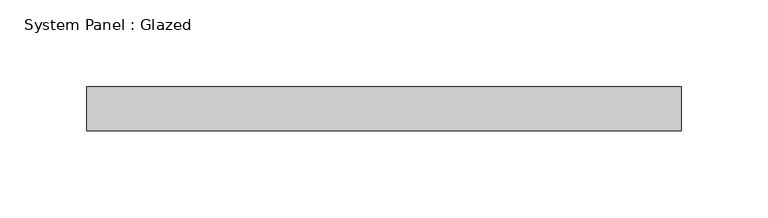
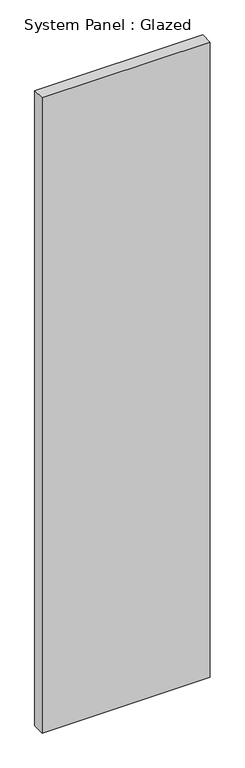
"""IFC4 building model written with IfcOpenShell, lengths in millimetres: plate geometry, System Panel : Glazed."""

from ifc_helpers import new_model, si_unit, origin, origin_with_axes, place, context, project, spatial, polyline, outline, extrude, source, transform, mapped, element, save


def system_panel_glazed_f11b7ff6(model_context):
    return source(origin(), model_context, "Body", "SweptSolid", [
        extrude(outline(polyline([(171.45, 19.05), (-171.45, 19.05), (-171.45, 44.45), (171.45, 44.45), (171.45, 19.05)])), origin_with_axes(), (0.0, 0.0, 1.0), 1368.5694058),
    ])


if __name__ == "__main__":
    model = new_model("IFC4")
    model_context = context("Model", 3, world=origin())
    ifc_project = project(units=[si_unit("LENGTHUNIT", "METRE", prefix="MILLI")], contexts=[model_context])
    site = spatial("IfcSite", under=ifc_project)
    building = spatial("IfcBuilding", under=site)
    placement = place(None, origin())
    system_panel_glazed_shape = system_panel_glazed_f11b7ff6(model_context)
    element("IfcPlate", 1, ObjectType="System Panel : Glazed", at=placement, inside=building, context=model_context, shape_type="MappedRepresentation", body=[
        mapped(system_panel_glazed_shape, transform((0.0, 0.0, 0.0), x_axis=(1.0, 0.0, 0.0), y_axis=(0.0, 1.0, 0.0), z_axis=(0.0, 0.0, 1.0))),
    ])
    save(model, "model.ifc")

# Revit data of these elements
# Type "System Panel : Glazed"
#   Construction Type Id = "GSP4R"
#   Analytic Construction = "1/8 in Pilkington single glazing"
#   Visual Light Transmittance = 0.9
#   Solar Heat Gain Coefficient = 0.86
#   Heat Transfer Coefficient (U) = 1.18115 BTU/(h·ft²·°F)
#   Define Thermal Properties by = 1
# Element 1 (IfcPlate, "System Panel : Glazed")
#   Materials on its faces: "Glass"
# Materials
#   "Glass": class "Glass", colour RGB 0 128 192, transparency 0.75, Description = "Soda Lime Glass", Cost = 0
